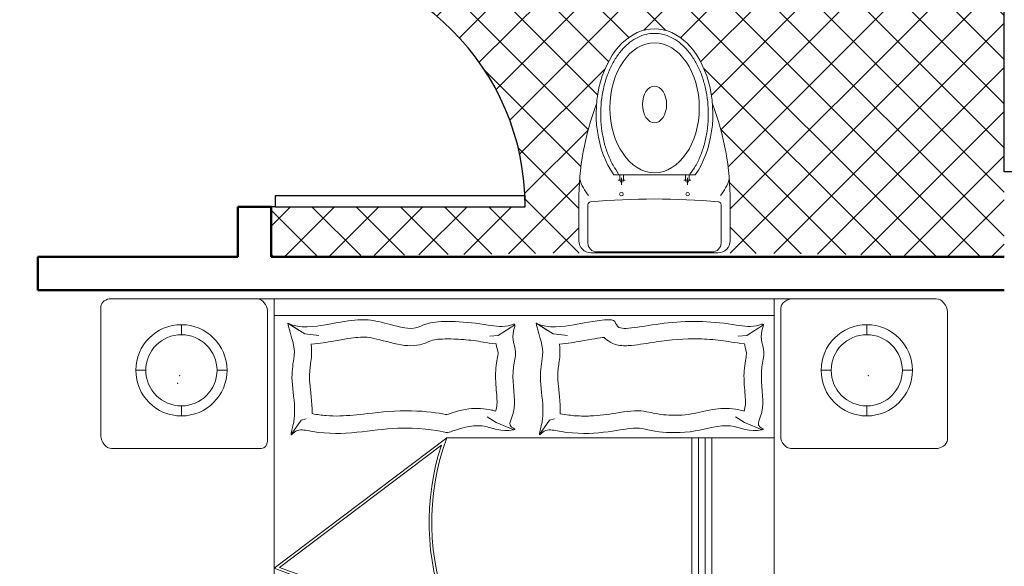
# Model space of a CAD drawing. Units: inches. Extents: x -466983 to 1020, y 324 to 318697.
# Tile 46 of 97: x 491 to 609, y 973 to 1038. Entities that reach past the tile are written whole.
import ezdxf

# ---------------------------------------------------------------- set-up
doc = ezdxf.new("R2010")
doc.units = ezdxf.units.IN
doc.header["$MEASUREMENT"] = 0
for name, color, linetype, lineweight in [('A-DOOR', 3, 'Continuous', 25), ('A-FLOR-FIXT', 9, 'Continuous', 18), ('A-FLOR-PATT', 252, 'Continuous', 13), ('A-FURN', 8, 'Continuous', 18), ('A-GLAZ', 4, 'Continuous', 25), ('A-WALL', 7, 'Continuous', 50)]:
    doc.layers.add(name, color=color, linetype=linetype, lineweight=lineweight)

# ---------------------------------------------------------------- blocks, each defined once
blk = doc.blocks.new('Ventilator')
for p, q in [((1433.5927409432, 801.6799676286266), (1457.592740943201, 801.6799676286266)), ((1433.5927409432, 792.6799676286266), (1433.5927409432, 801.6799676286266)), ((1457.592740943201, 801.6799676286266), (1457.592740943201, 792.6799676286266)), ((1433.5927409432, 797.9799676286265), (1457.592740943201, 797.9799676286265)), ((1457.592740943201, 796.3799676286266), (1433.5927409432, 796.3799676286266)), ((1457.592740943201, 792.6799676286266), (1433.5927409432, 792.6799676286266))]:
    blk.add_line(p, q)
blk = doc.blocks.new('A$C05F852CF')
for p, q in [((0.0305768516066087, 3.078317078245163), (0.4691515062860628, 3.078317078245164)), ((0.4691515062860671, 3.078317078245163), (2.07682031226372, 3.078317078245163)), ((0.5200001058256021, 3.078317078245163), (0.5200001058256021, 1.078317078245163)), ((2.020000105825602, 3.078317078245163), (2.020000105825602, 1.078317078245163)), ((2.076820312263923, 3.078317078245163), (2.506611773352182, 3.078317078245163)), ((1.058288035e-07, 3.054839612522671), (1.058288035e-07, 2.665863151727971)), ((2.040000105829676, 3.050045752684985), (2.040000105829677, 2.664204404880085)), ((0.5000001058288034, 3.042296501208146), (0.5000001058288035, 2.649646432748242)), ((0.5200001058256021, 3.028317078242253), (2.020000105825602, 3.028317078242253)), ((2.540000105829677, 2.654697021141195), (2.540000105829677, 3.039330964775836)), ((0.2417833150248043, 2.970224330108612), (0.2417833150248043, 3.000224330113269)), ((0.5608743282500654, 3.00448058915208), (0.5953432699752739, 2.982949469987943)), ((0.5608743282500654, 3.00448058915208), (0.6121479649955291, 2.972452371068357)), ((1.242739223729586, 2.999473446026968), (1.192734207375906, 2.968208048550877)), ((2.298216896626399, 2.970224330108612), (2.298216896626399, 3.000224330113269)), ((0.6121479649955291, 2.972452371068357), (0.6546239254166722, 2.968208048550877)), ((1.192734207375906, 2.968208048550877), (1.167248631121765, 2.9660858872885)), ((0.1349139653742895, 2.863354980458097), (0.1049139653742895, 2.863354980458097)), ((0.3486526646753191, 2.863354980458097), (0.3786526646753191, 2.863354980458097)), ((2.191347546975884, 2.863354980458097), (2.161347546975885, 2.863354980458097)), ((2.405086246276914, 2.863354980458097), (2.435086246276914, 2.863354980458097)), ((0.2417833150248043, 2.726485630810202), (0.2417833150248043, 2.756485630807583)), ((2.298216896626399, 2.726485630810202), (2.298216896626399, 2.756485630807583)), ((1.186362799460766, 2.707182858976011), (1.158753439034626, 2.724160116791608)), ((0.571055790554965, 2.671151427624863), (0.6015289887363906, 2.713549342755868)), ((0.6015289887363906, 2.713549342755868), (0.6163955887241173, 2.717793665280623)), ((1.239669649243296, 2.685196542661287), (1.186362799460766, 2.707182858976011)), ((1.037932771781925, 2.66077471069002), (0.5200001058256021, 2.269743772885703)), ((2.020000105825602, 2.66077471069002), (1.037932771781925, 2.66077471069002)), ((1.773666079527174, 2.66077471069002), (1.773666079527174, 1.078317078245163)), ((1.793666079523973, 2.66077471069002), (1.793666079523973, 1.078317078245163)), ((1.813666079528047, 2.66077471069002), (1.813666079528047, 1.078317078245163)), ((1.833666079524846, 2.66077471069002), (1.833666079524846, 1.078317078245163)), ((0.0321551649834042, 2.628317078240798), (0.4826422377176051, 2.628317078240797)), ((2.070734587595952, 2.628317078240797), (2.505643211553573, 2.628317078240797)), ((0.5200001058256021, 1.459699989092769), (2.020000105825602, 1.459699989092769)), ((0.5200001058256021, 1.43969998909597), (2.020000105825602, 1.43969998909597)), ((0.5200001058256021, 1.419699989099171), (2.020000105825602, 1.419699989099171)), ((0.5200001058256021, 1.399699989095097), (2.020000105825602, 1.399699989095097)), ((0.5200001058256021, 1.078317078245163), (2.020000105825602, 1.078317078245163)), ((0.7260346108741942, 0.4345828151708702), (0.7377091281887261, 0.4443788983408013))]:
    blk.add_line(p, q)
for points in [[(1.340512920731271, 2.982949469987943), (1.306043979006062, 3.00448058915208), (1.357317615751526, 2.972452371068357), (1.399793576172669, 2.968208048550877)], [(1.987908874485583, 2.999473446026968), (1.937903858124627, 2.968208048550877), (1.912418281870486, 2.9660858872885)], [(1.984839299999293, 2.685196542661287), (1.931532450216764, 2.707182858976011), (1.903923089790623, 2.724160116791608)], [(1.316225441310962, 2.671151427624863), (1.346698639485111, 2.713549342755868), (1.361565239480114, 2.717793665280623)]]:
    blk.add_lwpolyline(points)
for points in [[(1.035294798241981, 2.137877542112184, -0.1730319288328975), (1.021984534024188, 2.638847447216473), (0.5360171556477639, 2.271949793912513, 0.0538879536169309)], [(1.708050559093439, 1.775878924940549, 0.1013919188288575), (1.728157492045764, 1.750061837442286, -0.2237680031452591), (1.734490876633178, 1.736012066440117, -0.2555795276033393), (1.73151803809566, 1.730786319379855, -0.0815627079958122), (1.715055393804573, 1.724012337983466, -0.0718052278729777), (1.696654411599312, 1.722458737045573, 0.0699853124223817), (1.677774125455085, 1.720933512357767, 0.0354599114355874), (1.614797373554905, 1.702055242289732, 0.0294323486882548), (1.54253181370024, 1.669698476292178, 0.001553930981739), (1.507841381839936, 1.651508640737627, -0.0015200052493194), (1.472377942403747, 1.632910412866881, -0.0047351393002262), (1.435637173695639, 1.614224569329063, 0.003820482062427), (1.390058392027433, 1.591148680402633, 0.2960011454759293), (1.369157347081392, 1.554552950265695, -0.6497743315171824), (1.346832187453866, 1.543071524364048, -0.0231899320323143), (1.341607642712404, 1.547689019153187, 0.0288000576854015), (1.337358154039801, 1.551360714168372, 0.0057266563932194), (1.329792250482655, 1.557035683033763, -0.0043580795685463), (1.319830170733231, 1.564465434900571, -0.0275279631909796), (1.300139484251123, 1.581205024032326, -0.0462141900082825), (1.289988230316169, 1.592806604542285, -0.1941210974269485), (1.285597174805949, 1.61052060476509, 0.1337189317945981), (1.282347392942978, 1.636304919732166, 0.0115049885998871), (1.262248195883971, 1.682017285758821, 0.0088817842639035), (1.233822341202832, 1.740117109611183, 0.0124257132779513), (1.193744434042254, 1.813894083333623, -0.033612369588165), (1.180083210426986, 1.841797703870053), (1.155232457866077, 1.902584981879044), (1.136061875891755, 1.949478028393059, 0.224341071481397), (1.120380687047856, 1.963834925633848, -0.722771521635921), (1.120197630008879, 1.973398278848949, -0.1035130421165991), (1.124231807418808, 1.97393370871293, 0.0534647388739861), (1.132045497836501, 1.974187654123627, 0.0301092765073397), (1.156931902511403, 1.97921985894508, -0.0314364784170881), (1.180782283804338, 1.983976772955894, -0.0532399639377359), (1.197102041045038, 1.984427853473678, 0.0551795233422178), (1.212849660231511, 1.984924081265458, 0.0562710065808877), (1.240173079634912, 1.992022438719103, 0.0108003168714398), (1.37589919497303, 2.047527127645597, 0.0045599262081994), (1.467518199665537, 2.08832242005046, 0.0112502044116702), (1.504115679717903, 2.10602511197999, 0.0693939606021616), (1.523450236066789, 2.119584464602007, -0.0797562576808959), (1.540538561194231, 2.131050544499311, -0.1063994920026711), (1.556160884733792, 2.134540918040703, -0.3286420828127689), (1.560758069905846, 2.131208477514896, -0.2995467620412478), (1.558739430321109, 2.124014460027718, 0.1899166395855367), (1.553562506110245, 2.114077400326368, 0.0335175219245665), (1.553139912342055, 2.102935661711667, 0.0756271023396346), (1.554028972653962, 2.098051728963763, 0.0534886288518014), (1.55787110568871, 2.089846036281636, 0.0178378665464654), (1.572733087595266, 2.067184354551788, 0.0383935758418631), (1.593239248720917, 2.042483627130348, -0.0595290829391222), (1.605807381512724, 2.025975353424011, -0.0359425919331862), (1.619326798747338, 1.998683789839922, -0.0112450065700176), (1.654088856282072, 1.907874325597662, -0.006202709412992), (1.668419968066657, 1.866129904310976, 0.0107832106742137), (1.67688376537216, 1.842192375839789, 0.0194848354522239), (1.682775803493053, 1.828271519536226, 0.005061623460185)], [(1.695259182866416, 1.769547813629049, 0.0985872314327748), (1.718081561207793, 1.739905989662399, -0.0403778893328424), (1.71183503166025, 1.737916709378077, -0.0718052278729781), (1.697497903411904, 1.736706220956143, 0.0699853124223817), (1.674654559801433, 1.734860844706513, 0.0354599114355874), (1.609741097926352, 1.715402015419892, 0.0294323486882547), (1.535943288060523, 1.682359187414175, 0.001553930981739), (1.50117428856039, 1.664128155126926, -0.0015200052493194), (1.465787698753773, 1.645570229802914, -0.0047351393002262), (1.429287879954427, 1.627006930034647, 0.003820482062427), (1.383514509072797, 1.603832523357192, 0.2898135525162437), (1.354853178569346, 1.554951448117944, -0.0182793572286215), (1.35154491067881, 1.557933675398455, 0.0288000576854021), (1.346052337980832, 1.562679435024519, 0.0057266563932193), (1.338224905351514, 1.568550569402397, -0.0043580795685465), (1.328462264060592, 1.575831579409929, -0.0275279631909798), (1.309968032010976, 1.591554030030593, -0.0462141900082822), (1.301550432054356, 1.60117426653267, -0.1941210974269471), (1.299728996962296, 1.608522135660689, 0.1337189317945981), (1.295541371992653, 1.641747455267798, 0.0115049885998871), (1.275177841475791, 1.688061004902677, 0.0088817842639034), (1.246529163101812, 1.746616259820824, 0.0124257132779513), (1.206112688769413, 1.821016481189961, -0.0336123695881646), (1.193294292057559, 1.847198592534913), (1.168443539497244, 1.907985870542451), (1.149272957522402, 1.954878917057737, 0.0514173808819106), (1.145486925332716, 1.961962889445687, 0.0172081957648061), (1.160597165040831, 1.965426087640239, -0.031436478417088), (1.182689249433297, 1.969832312615894, -0.0532399639377359), (1.195979299991558, 1.970199651593374, 0.0551795233422181), (1.214865982280068, 1.970794795309813, 0.0562710065808877), (1.245288872283408, 1.978698364950264, 0.0108003168714398), (1.381585630304949, 2.034436416074573, 0.0045599262081997), (1.473442444961096, 2.075337598376756, 0.0112502044116702), (1.510618033905799, 2.093319929327427, 0.0693939606021616), (1.533180597587688, 2.109143088213213, -0.0381608677403329), (1.539212311339161, 2.113959948097047, 0.0293614558111777), (1.538873523984414, 2.102520403419968, 0.0756271023396326), (1.540531433152462, 2.093412903290674, 0.0534886288518001), (1.545664760729809, 2.082449589907588, 0.0178378665464654), (1.561085038110327, 2.058936614290585, 0.0383935758418633), (1.582989208528954, 2.032551912661889, -0.0595290829391216), (1.593505968643746, 2.018738122071704, -0.0359425919331862), (1.606115717130862, 1.99328290114058, -0.0112450065700176), (1.640648295649741, 1.903072908503876, -0.0062027094129919), (1.654864430545357, 1.861663397988524, 0.0107832106742138), (1.663533420481039, 1.837145538462979, 0.0194848354522239), (1.669858875879018, 1.822200666446777, 0.005061623460185)]]:
    blk.add_lwpolyline(points, format="xyb", close=True)
for points in [[(1.270020360572594, 1.665009431050252, 0.0256263766809095), (1.257496937469981, 1.661962907224936, 0.0108003168915285), (1.117915806080817, 1.617024549173869, 0.0045599250600183), (1.023439488402936, 1.583371629054553, 0.0112502042554101), (0.9855927851847837, 1.568526107768631, 0.0693939618380823), (0.9652758158050374, 1.556488585590853, -0.0797562567609452), (0.9473589151510481, 1.546366011015306, -0.1063994945831262), (0.9315150200727321, 1.5440833152102, -0.3286420812263602), (0.9271867815419792, 1.54775831472709, -0.2995467631228521), (0.9297508853421131, 1.554776445874623, 0.1899166395519681), (0.9356742299125951, 1.564287475604295, 0.0335175234261574), (0.9369495655297574, 1.575364047566859, 0.075627101586891), (0.9364374612317099, 1.580301757141754, 0.0534886298074961), (0.9332355752115681, 1.588777800893726, 0.0178378665269371), (0.9201542714773111, 1.612511950054128, 0.0383935757768284), (0.9016016807480021, 1.63871175657932, -0.0595290839550855), (0.8903358353981968, 1.656134782393036, -0.0359425913009802), (0.8789480177289066, 1.684382282033313, -0.0112450075583744), (0.8512485241325798, 1.777589041382892, -0.0062027096904869), (0.8401591725715132, 1.820309097441429, 0.0107832125180045), (0.8335550214589964, 1.844824938410538, 0.0194848341872523), (0.8287473142423458, 1.859156449308979, 0.0050616244400538), (0.8075626644720159, 1.913332163710765, 0.1013919188235688), (0.7894936926428668, 1.940614447702458, -0.22376800337822), (0.7842558173954927, 1.955108325059244, -0.2555795277823594), (0.7876204503391627, 1.960090839085296, -0.0815627097533239), (0.8045538741787872, 1.965583074885499, -0.0718052258191368), (0.8230198047757069, 1.965721718523918, 0.0699853122038087), (0.8419614541001006, 1.96579533206703, 0.0354599118842221), (0.9061999169328895, 1.979791065284685, 0.0294323472364991), (0.980732947874111, 2.006513679583421, 0.0015539321746028), (1.016715544742657, 2.021991080197058, -0.0015200050660023), (1.05350014010862, 2.037816406693342, -0.0047351399682821), (1.091565063355451, 2.053631204585071, 0.0038204811652429), (1.138778458583519, 2.07314571145658, 0.2960011456451315), (1.162422996298041, 2.10803178119455, -0.6497743308183526), (1.18556250232168, 2.117768267051117, -0.023189931893098), (1.190417758999585, 2.112763908071101, 0.0288000584975066), (1.194373321091643, 2.108777302019709, 0.0057266569232023), (1.201481997667391, 2.102539119626516, -0.0043580803905699), (1.210845298395146, 2.094367658855894, -0.0275279623196554), (1.229195014547529, 2.07616807397338, -0.046214191426687), (1.238427176317387, 2.063822554404071, -0.1941210967300704), (1.24144758291114, 2.045824101341992, 0.1337189329089291), (1.242711504870895, 2.019866549455296, 0.005779060601493), (1.250747094455965, 1.996102607779307)], [(1.267433777013181, 1.678650745174671, 0.0256263766809096), (1.25352836721457, 1.6752680308876, 0.0108003168915285), (1.113376341331941, 1.630145872481547, 0.0045599250600184), (1.018661464651108, 1.596407976494609, 0.0112502042554101), (0.9802331745365827, 1.581334325413979, 0.0693939618380822), (0.9566164053315807, 1.567341717664273, -0.0421754501329271), (0.9494714401999663, 1.562566648678462, 0.0314567403863147), (0.950818198592405, 1.574703076671485, 0.0756271015868911), (0.9498752735948789, 1.583794759352339, 0.0534886298074966), (0.9456266121275149, 1.595041830722721, 0.0178378665269371), (0.9320672656192937, 1.619643319917204, 0.0383935757768284), (0.9122842399252132, 1.647580735944291, -0.0595290839550849), (0.9028072117943391, 1.662237293051497, -0.0359425913009799), (0.8921648024522767, 1.688635806116587, -0.0112450075583744), (0.8646431932534301, 1.781243997565097, -0.006202709690487), (0.8536403913351593, 1.823630634163732, 0.0107832125180045), (0.8468804852507327, 1.848724666642867, 0.0194848341872522), (0.8417287394599854, 1.864081737612187, 0.0050616244400538), (0.8204417169625553, 1.918519250802461, 0.1002374450930622), (0.7996032399862063, 1.950139962323341, -0.0442087188515421), (0.806640704233721, 1.951856421765647, -0.0718052258191371), (0.8211393199436285, 1.951965278492165, 0.0699853122038086), (0.8439488047114903, 1.952053923729516, 0.0354599118842221), (0.910109066083358, 1.966468362162935, 0.0294323472364991), (0.9861794565215773, 1.993742171876655, 0.0015539321746028), (1.022241331845213, 2.00925367298648, -0.0015200050660023), (1.05894838186196, 2.025045638222023, -0.0047351399682822), (1.096770458708799, 2.040759540948764, 0.0038204811652431), (1.144179941304543, 2.06035509575735, 0.2942870031128779), (1.176296866445577, 2.107421377421802, -0.0218403622568167), (1.180015238936497, 2.103568069779355, 0.0288000584975063), (1.185096443349676, 2.098446987169159, 0.0057266569232022), (1.192444163039438, 2.091999033726075, -0.0043580803905699), (1.201625109260011, 2.083986715841735, -0.0275279623196552), (1.218890166936317, 2.066862915121399, -0.0462141914266873), (1.226588508356947, 2.05656846545553, -0.1941210967300651), (1.227889447910251, 2.048816231160124, 0.1337189329089299), (1.22950820338519, 2.015571354997711, 0.005779060601493), (1.237646599208447, 1.991503380689822, 0.005779060601493)]]:
    blk.add_lwpolyline(points, format="xyb")
for centre, radius in [((0.2417833150248043, 2.863354980458097), 0.1368693496505148), ((2.298216896626399, 2.863354980458097), 0.1368693496505148), ((0.2417833150248043, 2.863354980458097), 0.1068693496505148), ((2.298216896626399, 2.863354980458097), 0.1068693496505148)]:
    blk.add_circle(centre, radius)
for centre, radius, start, end in [((1.730780082035789, 2.407017656099047), 0.7378550251104214, 159.8846174586709, 202.2193637034114), ((1.40584522550477, 4.514464091946545), 2.413191017483698, 248.464074582217, 261.4655058976137)]:
    blk.add_arc(centre, radius, start, end)
for points in [[(1.058288035e-07, 3.054839612522671), (1.058288035e-07, 3.067689726137004), (0.0177267379922761, 3.078317078245163), (0.0305768516066087, 3.078317078245163)], [(0.5000001058288034, 3.042296501208146), (0.5000001058288034, 3.058104790397429), (0.4849597954753462, 3.078317078245164), (0.4691515062860628, 3.078317078245164)], [(2.040000105829676, 3.050045752684985), (2.040000105829676, 3.065519728870074), (2.061346336078835, 3.078317078245163), (2.076820312263923, 3.078317078245163)], [(2.506611773352182, 3.078317078245163), (2.523721542455991, 3.078317078245163), (2.540000105829677, 3.056440733879645), (2.540000105829677, 3.039330964775836)], [(0.0321551649834042, 2.628317078240798), (0.0156773837697008, 2.628317078240798), (1.058288035e-07, 2.649385370514268), (1.058288035e-07, 2.665863151727971)], [(2.040000105829677, 2.664204404880085), (2.040000105829677, 2.648454595065514), (2.05498477778138, 2.628317078240797), (2.070734587595952, 2.628317078240797)], [(0.5000001058288035, 2.649646432748242), (0.5000001058288035, 2.640479845178462), (0.4918088252873853, 2.628317078240797), (0.4826422377176051, 2.628317078240797)], [(2.505643211553573, 2.628317078240797), (2.52008196177545, 2.628317078240797), (2.540000105829677, 2.640258270919319), (2.540000105829677, 2.654697021141195)]]:
    blk.add_open_spline(points, degree=3)
for points, knots in [([(0.5608743282500654, 3.00448058915208), (0.5649926015757956, 2.981846978706016), (0.583561233303044, 2.936624526169907), (0.577615531939955, 2.888972981483675), (0.568850038027449, 2.835056739670108), (0.5831844526110217, 2.770926244731526), (0.5807655002863612, 2.708841986364859), (0.5743850803628447, 2.69267683673388), (0.5692655243474292, 2.665138401345757), (0.5802504519451759, 2.679294818459311), (0.5989340893502231, 2.687563487939769), (0.7172179605840939, 2.659836610568163), (0.8680758339905879, 2.702933271801157), (1.048422440333524, 2.678138835668505), (1.032371212037105, 2.673100819083629), (1.143052510538836, 2.711612612161843), (1.202032879395119, 2.675720859246212), (1.245920398971065, 2.686747608633595), (1.222151592133741, 2.694979075698938), (1.235874692996731, 2.725131493731169), (1.24678286496055, 2.780968112114351), (1.22880829625501, 2.849214346417284), (1.25148706651089, 2.925020729671814), (1.227919394332275, 2.960895142656227), (1.247080047731287, 3.005764387140516), (1.209778335498413, 2.990212765405885), (1.117656181813799, 3.009504931840638), (0.9559744755824794, 3.015881985804298), (0.9531522539109573, 2.975810997435473), (0.7998968530228013, 3.020986756855563), (0.7569283034463297, 3.015103121600986), (0.5985546251031338, 2.986850236149621), (0.5610488986203565, 3.004875976599578)], [16.81603238654801, 16.81603238654801, 16.81603238654801, 16.81603238654801, 79.03884518756725, 88.51389547092393, 147.5652660998466, 227.1968623982579, 259.6854484034709, 283.9553011869364, 296.5113041396114, 302.4325582064448, 320.2309418964503, 354.3225591584033, 575.2795485590284, 734.7235597353396, 845.7404214628034, 943.0331034920418, 1029.53396696452, 1032.845074190681, 1043.313583943025, 1065.311533561496, 1104.921834519419, 1208.530020162994, 1248.510714137047, 1303.102727458275, 1321.013260208933, 1329.647833410585, 1389.371623582993, 1571.817643787636, 1750.274160612537, 1823.189072856133, 1967.937032714809, 2020.91232922514, 2020.91232922514, 2020.91232922514, 2020.91232922514]), ([(1.306043979006062, 3.00448058915208), (1.310162252324516, 2.981846978706016), (1.328730884059041, 2.936624526169907), (1.322785182695952, 2.888972981483675), (1.31401968877617, 2.835056739670108), (1.328354103367018, 2.770926244731526), (1.325935151042358, 2.708841986364859), (1.319554731111566, 2.69267683673388), (1.31443517509615, 2.665138401345757), (1.325420102701173, 2.679294818459311), (1.344103740098944, 2.687563487939769), (1.462387611340091, 2.659836610568163), (1.613245484739309, 2.702933271801157), (1.643592091088066, 2.678138835668505), (1.777540862793102, 2.673100819083629), (1.888222161287558, 2.711612612161843), (1.947202530151116, 2.675720859246212), (1.991090049727063, 2.686747608633595), (1.967321242889738, 2.694979075698938), (1.981044343745452, 2.725131493731169), (1.991952515709272, 2.780968112114351), (1.973977947003731, 2.849214346417284), (1.996656717266887, 2.925020729671814), (1.973089045080996, 2.960895142656227), (1.992249698480009, 3.005764387140516), (1.95494798625441, 2.990212765405885), (1.862825832569797, 3.009504931840638), (1.7011441263312, 3.015881985804298), (1.548321904665499, 2.975810997435473), (1.545066503778798, 3.020986756855563), (1.502097954202326, 3.015103121600986), (1.343724275859131, 2.986850236149621), (1.306218549376353, 3.004875976599578)], [16.81603238654801, 16.81603238654801, 16.81603238654801, 16.81603238654801, 79.03884518756725, 88.51389547092393, 147.5652660998466, 227.1968623982579, 259.6854484034709, 283.9553011869364, 296.5113041396114, 302.4325582064448, 320.2309418964503, 354.3225591584033, 575.2795485590284, 734.7235597353396, 845.7404214628034, 943.0331034920418, 1029.53396696452, 1032.845074190681, 1043.313583943025, 1065.311533561496, 1104.921834519419, 1208.530020162994, 1248.510714137047, 1303.102727458275, 1321.013260208933, 1329.647833410585, 1389.371623582993, 1571.817643787636, 1750.274160612537, 1823.189072856133, 1967.937032714809, 2020.91232922514, 2020.91232922514, 2020.91232922514, 2020.91232922514]), ([(1.186008792049375, 2.94299214351074), (1.155725921251891, 2.945585073046202), (1.138656601401412, 2.950208126398367), (1.097630905252152, 2.95509280500171), (1.077589870855775, 2.956659449204214), (1.034238225660662, 2.958226127717206), (1.012323327727554, 2.957004601752403), (0.991001711516253, 2.953273250088436), (0.9901760228479028, 2.951676768007356), (0.9620368334136054, 2.940252037519872), (0.9370877461655887, 2.935037325494899), (0.8850511336414232, 2.94132938915891), (0.8522462034232987, 2.951314821397172), (0.803295939310399, 2.96285187557315), (0.7937503361772829, 2.963996187832593), (0.7550144806336718, 2.960828646016758), (0.7318586182640057, 2.957210255508529), (0.679441891670091, 2.948089555791339), (0.6579881949560275, 2.943409279898279), (0.630985700249326, 2.941762475625111)], [1364.380335490081, 1364.380335490081, 1364.380335490081, 1364.380335490081, 1423.602309547691, 1423.602309547691, 1482.824283605301, 1482.824283605301, 1566.205036495643, 1566.205036495643, 1649.585789385986, 1649.585789385986, 1732.966542276328, 1732.966542276328, 1816.347295166671, 1816.347295166671, 1899.728048057014, 1899.728048057014, 1960.499853060085, 1960.499853060085, 1990.525565429441, 1990.525565429441, 1990.525565429441, 1990.525565429441]), ([(1.510355574678164, 2.962131737273937), (1.496402554093968, 2.960566078706099), (1.473180590099924, 2.956790270249104), (1.422578285991909, 2.947958552952412), (1.401696155951149, 2.943524922981268), (1.375888251815216, 2.941975038078444)], [1904.396500054124, 1904.396500054124, 1904.396500054124, 1904.396500054124, 1961.927875749907, 1961.927875749907, 1990.619444948187, 1990.619444948187, 1990.619444948187, 1990.619444948187]), ([(1.931373767935067, 2.94320464204133), (1.899671311434888, 2.945891083962288), (1.88221689097919, 2.950718490397115), (1.838682954929346, 2.955652880867252), (1.816795986262647, 2.957169928676467), (1.751472258998956, 2.958725448706285), (1.708807917427409, 2.955142722863579), (1.640333479281332, 2.944746536498916), (1.615392287461663, 2.940198542969911), (1.579493331147493, 2.936988078909458), (1.567546271042127, 2.936091768500583), (1.539405034045934, 2.941198470052663), (1.5201082499519, 2.950733332609488), (1.510355574678187, 2.962131737273942)], [1364.265661087181, 1364.265661087181, 1364.265661087181, 1364.265661087181, 1426.240794565023, 1426.240794565023, 1488.215928042865, 1488.215928042865, 1612.166194998548, 1612.166194998548, 1689.928639661805, 1689.928639661805, 1733.064361503359, 1733.064361503359, 1768.978829433574, 1768.978829433574, 1768.978829433574, 1768.978829433574]), ([(0.6309857002492723, 2.941762475624982), (0.6331564334752285, 2.928751157475458), (0.6329999809455203, 2.910376883670986), (0.6307844219696133, 2.892950992011628), (0.6298480683836976, 2.88648431095065), (0.6280366860877277, 2.872562196049626), (0.6272625999342161, 2.865990559597485), (0.6256841353987236, 2.847428671628844), (0.6257494163208535, 2.83751285108547), (0.6289829528156191, 2.801318580102345), (0.6345320734627763, 2.769590933476876), (0.6337228367630585, 2.733309880517507)], [67.28536243525942, 67.28536243525942, 67.28536243525942, 67.28536243525942, 87.39955824583018, 87.39955824583018, 107.5137540564009, 107.5137540564009, 127.6279498669717, 127.6279498669717, 167.8563414881131, 167.8563414881131, 238.1272680512623, 238.1272680512623, 238.1272680512623, 238.1272680512623]), ([(1.184532074545908, 2.741151129000606), (1.18898166794339, 2.755206550563011), (1.189354860725254, 2.765005834716451), (1.187413425890239, 2.799822569981758), (1.184324887423806, 2.821896583953417), (1.184425468230181, 2.866418567383826), (1.188231061791394, 2.890075729955087), (1.192008110665926, 2.910542534993727), (1.192192726159281, 2.914423416697752), (1.192086062290282, 2.915789359669391), (1.190808194988107, 2.921220065210955), (1.187543579250811, 2.935072419567428), (1.18672591971923, 2.938807649824122), (1.186008792049374, 2.94299214351074)], [1072.516900511537, 1072.516900511537, 1072.516900511537, 1072.516900511537, 1129.100963921242, 1129.100963921242, 1185.685027330947, 1185.685027330947, 1226.035089289856, 1226.035089289856, 1249.281274409203, 1249.281274409203, 1272.52745952855, 1272.52745952855, 1279.68927491123, 1279.68927491123, 1279.68927491123, 1279.68927491123]), ([(1.375888251815172, 2.941975038078342), (1.378074137039331, 2.928979344370601), (1.377968860976706, 2.910637565443015), (1.375735790312178, 2.893015133736763), (1.37480390116772, 2.88660606446792), (1.37298778010343, 2.872656318465669), (1.37221091417058, 2.866070180858095), (1.370625496709551, 2.847462614183982), (1.370689547662139, 2.837514257962978), (1.37393087155791, 2.801238188465308), (1.379492518843283, 2.769438786188064), (1.378659813172273, 2.733119478683537)], [67.15622801377181, 67.15622801377181, 67.15622801377181, 67.15622801377181, 87.29721209066957, 87.29721209066957, 107.4381961675674, 107.4381961675674, 127.5791802444651, 127.5791802444651, 167.8611483982607, 167.8611483982607, 238.2535697831694, 238.2535697831694, 238.2535697831694, 238.2535697831694]), ([(1.929853198197663, 2.740873894614667), (1.934365908758641, 2.755026217031627), (1.934751701761907, 2.764815030887031), (1.932835938875, 2.79960316592369), (1.929746498563042, 2.821657635936312), (1.929805814653183, 2.866185379441856), (1.933600746470114, 2.88991221701699), (1.937403886615359, 2.910503728082434), (1.937594356706148, 2.914393286831795), (1.937478304969509, 2.915863471904236), (1.936169207211093, 2.921368445863724), (1.93289467066463, 2.935308900229952), (1.932083262228118, 2.939035512649967), (1.931373767950089, 2.943204642135211)], [1072.238498285051, 1072.238498285051, 1072.238498285051, 1072.238498285051, 1128.864868567103, 1128.864868567103, 1185.491238849155, 1185.491238849155, 1225.989552664987, 1225.989552664987, 1249.32640120519, 1249.32640120519, 1272.663249745394, 1272.663249745394, 1279.788507909373, 1279.788507909373, 1279.788507909373, 1279.788507909373]), ([(1.03809723815708, 2.73039727020292), (1.049717200660217, 2.734487788763535), (1.074192496521652, 2.74352113186204), (1.125142067689975, 2.75041210718968), (1.152757231246774, 2.748989383813843), (1.176896856726861, 2.743194484257486), (1.18086569021346, 2.742138176736147), (1.184532074545908, 2.741151129000606)], [843.6450298341101, 843.6450298341101, 843.6450298341101, 843.6450298341101, 911.2757195712669, 911.2757195712669, 959.0880622759533, 959.0880622759533, 969.4799795511734, 969.4799795511734, 969.4799795511734, 969.4799795511734]), ([(1.37865981314566, 2.733119478685147), (1.398350924522489, 2.729609953669208), (1.410621471748096, 2.727818570031879), (1.440144629954641, 2.725836663619492), (1.45453272438222, 2.72579428596297), (1.496194066974801, 2.72756283296527), (1.521854810648972, 2.731279274356243), (1.576694937727594, 2.739864181267917), (1.6067435507169, 2.743633804836029), (1.652654114968593, 2.737068097937112), (1.661975420857501, 2.732604969096766), (1.708415029150631, 2.728170445544914), (1.736441496722281, 2.727579800786222), (1.784873006914288, 2.733957286540809), (1.807601793062205, 2.740559362958333), (1.856301372606796, 2.748907303561592), (1.881197134759921, 2.750793202553537), (1.914047432134626, 2.745130255701714), (1.922553922867449, 2.74284011529716), (1.929853198197665, 2.74087389461467)], [345.2679180365509, 345.2679180365509, 345.2679180365509, 345.2679180365509, 387.1674142554489, 387.1674142554489, 429.0669104743468, 429.0669104743468, 512.8659029121428, 512.8659029121428, 629.3175453119198, 629.3175453119198, 745.7691877116971, 745.7691877116971, 834.6228130435273, 834.6228130435273, 901.4144086089123, 901.4144086089123, 948.9218778206058, 948.9218778206058, 969.6795111477606, 969.6795111477606, 969.6795111477606, 969.6795111477606]), ([(0.6337228367630439, 2.733309880517508), (0.6515219447508598, 2.730130838331354), (0.6627469292146047, 2.728404560298634), (0.6898215070493534, 2.726294045804654), (0.7032356687061024, 2.726036490933712), (0.7435886058342663, 2.726989827329198), (0.7706550133649461, 2.729971405875143), (0.8408783579177043, 2.738316880491805), (0.888120323933067, 2.743221924747295), (0.9755155714750383, 2.740575358042937), (1.012451770127618, 2.735676002774785), (1.035649434709067, 2.730930674356534), (1.036885983111078, 2.730667355489783), (1.038097238090126, 2.730397270179416)], [345.40469962997, 345.40469962997, 345.40469962997, 345.40469962997, 383.3860561782741, 383.3860561782741, 421.3674127265782, 421.3674127265782, 497.3301258231863, 497.3301258231863, 611.5614694743621, 611.5614694743621, 725.792813125538, 725.792813125538, 732.4347682895597, 732.4347682895597, 732.4347682895597, 732.4347682895597])]:
    blk.add_open_spline(points, degree=3, knots=knots)
for p in [(0.2366049805932562, 2.847463833648362), (2.303395231057947, 2.847463833648362), (0.2308577250878443, 2.824418416894332), (2.020000105825602, 1.078317078245163), (2.020000105825602, 1.078317078245163)]:
    blk.add_point(p)
blk = doc.blocks.new('A$C005B7AE8')
for p, q in [((0.4599999173160541, 0.7399999669141835), (0.0399999173159813, 0.7399999669141835)), ((0.439999917316527, 0.7369231961274636), (0.0599999173164179, 0.7369231961274636)), ((-8.26839823e-08, 0.6999999669133103), (-8.26839823e-08, 0.5690287834004267)), ((0.0299999173166725, 0.7069231961286278), (0.029999917315763, 0.5811477270617617)), ((0.4699999173162724, 0.7069231961286278), (0.4699999173162724, 0.5811477270617617)), ((0.4999999173160177, 0.6999999669133103), (0.4999999173160177, 0.5690287833785987)), ((0.1298495880610062, 0.5003783992360696), (0.1533971911394474, 0.5003783992360696)), ((0.135565754210802, 0.4819999669125537), (0.135565754210802, 0.5011511907214299)), ((0.1415172819179133, 0.4916755243175431), (0.1415172819179133, 0.5154492432702682)), ((0.1478168830781215, 0.5011511907214299), (0.1478168830781215, 0.4819999669125537)), ((0.3701502465710291, 0.5003783992360696), (0.3466026434934974, 0.5003783992360696)), ((0.3521829515548234, 0.5011511907214299), (0.3521829515548234, 0.4819999669125537)), ((0.3584825527150315, 0.4916755243175431), (0.3584825527150315, 0.5154492432702682)), ((0.3644340804221429, 0.4819999669125537), (0.3644340804221429, 0.5011511907214299)), ((0.3846918195813487, 0.4819999669125537), (0.1153080150515962, 0.4819999669125537))]:
    blk.add_line(p, q)
for centre in [(0.1407590817070741, 0.546016981927096), (0.3592407529249613, 0.546016981927096)]:
    blk.add_circle(centre, 0.0058207128015492)
for centre, radius, start, end in [((0.0399999173159813, 0.6999999669133103), 0.04, 90, 180), ((0.0599999173164179, 0.7069231961286278), 0.03, 90, 180), ((0.439999917316527, 0.7069231961286278), 0.03, 0, 90), ((0.4599999173160541, 0.6999999669133103), 0.04, 0, 90), ((0.9162347733818023, 0.5697843573143473), 0.9162351676084766, 179.9527510438183, 200.6123382500767), ((0.0399999173159813, 0.5811477270617617), 0.01, 180, 265.0114580301616), ((0.2499999173160177, 2.986999966909934), 2.424999999999394, 265.0114580301616, 274.9885419698384), ((-0.4162349387497671, 0.5697843573143473), 0.9162351676084766, 339.3876617499233, 0.0472489561816761), ((0.4599999173160541, 0.5811477270617617), 0.01, 274.9885419698384, 0), ((0.1538218116911594, 0.4497837234594045), 0.1578971577643038, 140.181504794802, 162.8477667450203), ((0.346178022940876, 0.4497837234594045), 0.1578971577643038, 17.15223325497964, 39.81849520519793), ((0.141691318644007, 0.5005983719747747), 0.0061504591858251, 5.156848388262675, 174.8431516117373), ((0.3583085159880284, 0.5005983719747747), 0.0061504591858251, 5.156848388262675, 174.8431516117373)]:
    blk.add_arc(centre, radius, start, end)
blk.add_ellipse((0.2499999173160177, 0.2809999669116223), major_axis=(4.3e-15, -0.2809999999999999), ratio=0.6859192225533541, start_param=3.915332106759934, end_param=8.65103850759918)
for centre, major_axis, ratio in [((0.2497273054386824, 0.2607283879333408), (4.6e-15, -0.2143896387416461), 0.687861093389952), ((0.2499999173160177, 0.2495750337038771), (4e-16, -0.0607231097518234), 0.6571642650459009)]:
    blk.add_ellipse(centre, major_axis=major_axis, ratio=ratio)
blk.add_open_spline([(0.1330304284401791, 0.4805691871661111), (0.123297561966865, 0.467275065217109), (0.1192040598116364, 0.4608387557527749), (0.1089923119561718, 0.4430896997000673), (0.103240873932009, 0.4312752909245319), (0.0930943572666365, 0.4063656141879619), (0.0886993987696769, 0.3932708291395102), (0.0814055876480779, 0.3661625228414778), (0.0785067868491751, 0.352149423713854), (0.0742960000825406, 0.3235936370911077), (0.0729840366493591, 0.3090513401839416), (0.0719875980385041, 0.2798412472329801), (0.0723031276866095, 0.2651738304266473), (0.0745519352649353, 0.2361210512899561), (0.076485202062031, 0.2217360707581975), (0.0819094268572371, 0.1936478195857489), (0.0854003532995194, 0.1799449487807578), (0.0938301373234936, 0.1536010168056237), (0.0987689237617815, 0.1409603975334903), (0.1099364044266622, 0.1170889910499682), (0.116164929732804, 0.1058587174047716), (0.1297089136187424, 0.0851097239210503), (0.1370239707930523, 0.0755915829504375), (0.152501027386279, 0.0585057705757208), (0.1606621934961367, 0.0509385682526045), (0.1775722209031301, 0.0379140469667618), (0.1863198251348876, 0.0324565718765371), (0.2041561746218576, 0.023724375780148), (0.2132440667546689, 0.0204483489505947), (0.2315630702087219, 0.0160859502211679), (0.2407950771003016, 0.01499791808601), (0.259256859623747, 0.0150020215223776), (0.2684887415816775, 0.0160941591893789), (0.2868071874390807, 0.0204647859718534), (0.2958946431490403, 0.0237449365959037), (0.3137296967424845, 0.0324853214769974), (0.3224764393571604, 0.0379468595056096), (0.3393842548493922, 0.0509792925877264), (0.3475440710253679, 0.058550341942464), (0.3630179485271583, 0.0756434699942474), (0.3703311774997928, 0.0851650790282293), (0.3838710834670564, 0.1059204943594523), (0.3900973596782933, 0.1171537218178855), (0.4012600005589775, 0.1410304195233039), (0.4061961965880983, 0.1536733763350639), (0.4146205471060967, 0.1800212940433994), (0.4181086305634381, 0.1937258131365524), (0.423527009337704, 0.2218166234742966), (0.425457273147913, 0.2362025149268447), (0.4277000090169168, 0.2652563529190957), (0.4280124699726003, 0.2799239176820265), (0.427009923148944, 0.3091335394783528), (0.4256949202253964, 0.3236752172670094), (0.4214781782784485, 0.3522290158871328), (0.4185764618305257, 0.3662407460942632), (0.4112770365782126, 0.3933456040758756), (0.406879379678685, 0.4064383096483653), (0.3967277738520352, 0.4313431800474064), (0.3909739452683425, 0.4431548618158559), (0.380770586511062, 0.4608783582370961), (0.376689084062491, 0.467293849651469), (0.3673029200963356, 0.4823032274071011)], degree=3, knots=[3.915332106759953, 3.915332106759953, 3.915332106759953, 3.915332106759953, 4.014440589322762, 4.014440589322762, 4.176504673233075, 4.176504673233075, 4.338568757143389, 4.338568757143389, 4.500632841053702, 4.500632841053702, 4.662696924964015, 4.662696924964015, 4.824761008874329, 4.824761008874329, 4.986825092784642, 4.986825092784642, 5.148889176694956, 5.148889176694956, 5.310953260605269, 5.310953260605269, 5.473017344515582, 5.473017344515582, 5.635081428425896, 5.635081428425896, 5.797145512336209, 5.797145512336209, 5.959209596246522, 5.959209596246522, 6.121273680156836, 6.121273680156836, 6.283337764067149, 6.283337764067149, 6.445401847977462, 6.445401847977462, 6.607465931887776, 6.607465931887776, 6.769530015798089, 6.769530015798089, 6.931594099708402, 6.931594099708402, 7.093658183618716, 7.093658183618716, 7.255722267529029, 7.255722267529029, 7.417786351439342, 7.417786351439342, 7.579850435349656, 7.579850435349656, 7.741914519259969, 7.741914519259969, 7.903978603170283, 7.903978603170283, 8.066042687080596, 8.066042687080596, 8.22810677099091, 8.22810677099091, 8.390170854901225, 8.390170854901225, 8.552234938811539, 8.552234938811539, 8.651038507599205, 8.651038507599205, 8.651038507599205, 8.651038507599205])
blk = doc.blocks.new('*U38')
for p, q in [((0, 0), (-1.1e-15, 5.999999999999999)), ((40, 8e-15), (40, 6.000000000000007))]:
    blk.add_line(p, q)
blk.add_lwpolyline([(0, 0), (1.42e-14, -40), (1.750000000000014, -40), (1.75, 9e-16)], close=True)
blk.add_arc((0, 0), 40, 270, 0)

msp = doc.modelspace()

# ---------------------------------------------------------------- hatches: boundary and pattern name
at = {"layer": 'A-FLOR-PATT', "transparency": 33554572}
h = msp.add_hatch(dxfattribs=at)
h.set_pattern_fill('ANSI37', color=256, scale=30)
h.set_pattern_definition([(45, (-1212.413693079869, -290.0350025265127), (-2.651650429449553, 2.651650429449553), []), (135, (-1212.413693079869, -290.0350025265127), (-2.651650429449553, -2.651650429449552), [])])
h.paths.add_polyline_path([(901.805677520904, 1075.937732818422), (900.6144036774049, 1075.937732818422), (900.6144036774049, 1065.385628316983), (899.390971271441, 1065.385628316983), (898.0910743401043, 1065.385628316983), (892.8355944880973, 1058.709752245277, -0.2583770168556315), (892.18750428989, 1058.350891982691), (879.9847834232776, 1058.350891982691, -0.2017697719240963), (879.438188978411, 1058.580825279484), (874.0812133730635, 1065.385628316983), (872.7813164417267, 1065.385628316983), (871.5578840357629, 1065.385628316983), (871.5578840357629, 1075.937732818422), (813.8056775209042, 1075.937732818422), (813.8056775209042, 1044.792233318721), (832.3947444543938, 1044.792233318721, -0.3947951267487684), (848.6601780212009, 1028.535584015862), (848.6601780212009, 1009.937732818421), (901.805677520904, 1009.937732818421), (901.805677520904, 1015.937732818421), (901.3056775209042, 1015.937732818421), (871.3056775209039, 1015.937732818421), (871.3056775209039, 1017.250232818421), (871.3344022102003, 1017.250232818421, -0.4014527144963572), (901.3056775209042, 1045.937732818421), (901.805677520904, 1045.937732818421)])
edge = h.paths.add_edge_path(flags=16)
edge.add_line((847.7730719745084, 1068.948588737025), (847.7730719745069, 1073.708823774771))
edge.add_arc((849.2268986539951, 1073.708823774771), 1.453826679487974, 90, 180, ccw=False)
edge.add_line((849.2268986539951, 1075.162650454259), (864.4920787886183, 1075.162650454259))
edge.add_arc((864.4920787886213, 1073.708823774771), 1.453826679487974, 0, 90.00000000012102, ccw=False)
edge.add_line((865.9459054681093, 1073.708823774771), (865.9459054681081, 1069.00351244647))
edge.add_arc((832.6447385074767, 1068.976050591752), 33.30117828385809, -20.61233806670998, 0.04724903539101888, ccw=False)
edge.add_ellipse((856.8594887213083, 1058.479989307073), major_axis=(-2.091e-13, 10.21313242340307), ratio=0.6859192225533502, start_angle=100.00884331843292, end_angle=259.9911566815624, ccw=False)
edge.add_arc((881.0742389351396, 1068.976050591752), 33.30117828385809, 180.0472490354062, 200.6123380667097, ccw=False)
h.paths.add_polyline_path([(853.145578187156, 1066.481532374271), (853.145578187156, 1066.453444752512), (853.1463399851561, 1066.453444752512, 0.4331071439582673), (852.9166149812349, 1066.684892837266), (852.9166149812349, 1066.453444752512), (853.145578187156, 1066.453444752512), (853.145578187156, 1066.481532374489), (853.088019486549, 1066.612171966583, 0.6979386910037918), (852.699540939094, 1066.453444752512), (852.7003027371272, 1066.453444752512), (852.7003027371272, 1066.481532374489), (852.9166149812349, 1067.001204630995), (852.9166149812349, 1066.684892837266, -0.3962543063594317)], flags=0)
h.paths.add_polyline_path([(861.0186747055222, 1066.481532374271), (861.0186747055222, 1066.453444752512), (861.0194365035225, 1066.453444752512, 0.4164039232557909), (860.8023624614146, 1066.684892837265), (860.8023624614146, 1066.453444752512), (861.0186747055222, 1066.453444752512), (861.0186747055222, 1066.481532374489), (860.9671752720659, 1066.605255499379, 0.7133437187663149), (860.5726374574602, 1066.453444752512), (860.5733992554934, 1066.453444752512), (860.5733992554934, 1066.481532374489), (860.8023624614146, 1067.001204630995), (860.8023624614146, 1066.684892837265, -0.3799725304814568)], flags=0)
edge = h.paths.add_edge_path(flags=0)
edge.add_spline(control_points=[(861.1298377106021, 1065.785468371534), (861.4660965533383, 1065.247811229462), (861.613385559155, 1065.016139861057), (861.9832837951076, 1064.373617117607), (862.1924105327118, 1063.944313665492), (862.5613774174725, 1063.039129539609), (862.7212131906668, 1062.56326642291), (862.9865156700853, 1061.578122280975), (863.0919804897928, 1061.068856600952), (863.2452407883674, 1060.031049745086), (863.293035446714, 1059.502522766744), (863.3294736797056, 1058.440879580113), (863.3181170778639, 1057.907777155726), (863.2366033468288, 1056.85179603536), (863.1664466211855, 1056.328931215311), (862.9695120306455, 1055.307951977375), (862.8427353108815, 1054.809852090196), (862.5365466723708, 1053.852219447362), (862.3571373353129, 1053.392702749349), (861.9514237071658, 1052.524888245794), (861.7251255454219, 1052.116609101398), (861.2330086320977, 1051.362239687588), (860.9672044472572, 1051.016170456457), (860.4047960485765, 1050.394909316517), (860.1082220871676, 1050.119734477926), (859.493696255806, 1049.64606200509), (859.1757900615103, 1049.447558762665), (858.5275631429041, 1049.129883644436), (858.197273503909, 1049.010664382187), (857.5314773710529, 1048.851811036626), (857.1959384637446, 1048.812116564677), (856.5249326641573, 1048.811967422545), (856.1893892160524, 1048.851512676201), (855.5235728169741, 1049.010066967686), (855.1932673158994, 1049.129136347874), (854.5449932971788, 1049.446513839261), (854.2270557868354, 1049.644869411481), (853.6124495619564, 1050.118254324803), (853.3158265363004, 1050.393289340464), (852.7533025914207, 1051.014284587242), (852.487431959371, 1051.360227769297), (851.9951668313728, 1052.114363776776), (851.7687869247744, 1052.522535562859), (851.3628973914427, 1053.390157753425), (851.1833939042357, 1053.849589492002), (850.8770077813263, 1054.807077270704), (850.7501277313783, 1055.30511724975), (850.5529806633081, 1056.326003473117), (850.4827147921034, 1056.848835185142), (850.4009803807432, 1057.904777820697), (850.3895122452288, 1058.437874867502), (850.425728471152, 1059.499535178563), (850.4734126571939, 1060.02808465918), (850.6264565107679, 1061.065963770327), (850.7318153592672, 1061.575279204679), (850.9969137893603, 1062.560548677974), (851.1566514873134, 1063.036487374614), (851.525433403113, 1063.94184619004), (851.7344732542367, 1064.371248757046), (852.1056260411488, 1065.016350037675), (852.2544071072941, 1065.250281998093), (852.608154630964, 1065.733465727338)], knot_values=[3.915332106759953, 3.915332106759953, 3.915332106759953, 3.915332106759953, 4.013467662305501, 4.013467662305501, 4.175531746215815, 4.175531746215815, 4.337595830126129, 4.337595830126129, 4.499659914036444, 4.499659914036444, 4.661723997946757, 4.661723997946757, 4.82378808185707, 4.82378808185707, 4.985852165767384, 4.985852165767384, 5.147916249677697, 5.147916249677697, 5.30998033358801, 5.30998033358801, 5.472044417498324, 5.472044417498324, 5.634108501408637, 5.634108501408637, 5.79617258531895, 5.79617258531895, 5.958236669229264, 5.958236669229264, 6.120300753139577, 6.120300753139577, 6.282364837049891, 6.282364837049891, 6.444428920960204, 6.444428920960204, 6.606493004870517, 6.606493004870517, 6.768557088780831, 6.768557088780831, 6.930621172691144, 6.930621172691144, 7.092685256601457, 7.092685256601457, 7.254749340511771, 7.254749340511771, 7.416813424422084, 7.416813424422084, 7.578877508332397, 7.578877508332397, 7.740941592242711, 7.740941592242711, 7.903005676153024, 7.903005676153024, 8.065069760063338, 8.065069760063338, 8.22713384397365, 8.22713384397365, 8.389197927883965, 8.389197927883965, 8.551262011794279, 8.551262011794279, 8.650370494357087, 8.650370494357087, 8.650370494357087, 8.650370494357087], degree=3, periodic=0)
edge.add_line((852.6421178657537, 1065.785468371534), (861.1298377106024, 1065.785468371534))
edge = h.paths.add_edge_path(flags=0)
edge.add_ellipse((856.8495804607978, 1057.743205248224), major_axis=(-3.1e-13, 7.792134415209829), ratio=0.6878610933899516, start_angle=0, end_angle=360)
h.paths.add_polyline_path([(848.8634419841151, 1069.389059844444), (848.863441984139, 1073.960453158315, -0.4142135623709757), (849.9538119937549, 1075.050823167924), (863.765165448898, 1075.050823167924, -0.4142135623721942), (864.8555354585106, 1073.960453158308), (864.8555354584933, 1069.389059844444, -0.3889362887010341), (864.5236837164459, 1069.026979909221, -0.0435607626104464), (849.19529372618, 1069.02697990933, -0.3889362886276668)], flags=0)
h.paths.add_polyline_path([(853.1006153779753, 1068.112209480768, -1), (852.677499999749, 1068.112209480768, -1)], flags=0)
edge = h.paths.add_edge_path(flags=0)
edge.add_ellipse((856.8594887213083, 1057.33782914961), major_axis=(7.74e-14, 2.20702192546696), ratio=0.6571642650458812, start_angle=0, end_angle=360)
h.paths.add_polyline_path([(861.0414774428674, 1068.112209480768, -1), (860.6183620646412, 1068.112209480768, -1)], flags=0)
edge = h.paths.add_edge_path()
edge.add_line((573.9536545579417, 1057.341203598636), (573.9536545579417, 1075.937732818422))
edge.add_line((573.9536545579417, 1075.937732818422), (558.7307922536265, 1075.937732818422))
edge.add_line((558.7307922536265, 1075.937732818422), (558.7307922536265, 1065.385628316983))
edge.add_line((558.7307922536265, 1065.385628316983), (557.5073598476627, 1065.385628316983))
edge.add_line((557.5073598476627, 1065.385628316983), (556.207462916326, 1065.385628316983))
edge.add_line((556.207462916326, 1065.385628316983), (550.9519830643189, 1058.709752245277))
edge.add_arc((550.3038928661116, 1059.115537236419), 0.7646452537275144, 270, 327.94831933647396, ccw=False)
edge.add_line((550.3038928661116, 1058.350891982691), (538.1011719994992, 1058.350891982691))
edge.add_arc((538.1011719994992, 1059.115537236419), 0.7646452537275137, 224.3704013916024, 270, ccw=False)
edge.add_line((537.5545775546327, 1058.580825279484), (532.1976019492852, 1065.385628316983))
edge.add_line((532.1976019492852, 1065.385628316983), (530.8977050179485, 1065.385628316983))
edge.add_line((530.8977050179485, 1065.385628316983), (529.6742726119846, 1065.385628316983))
edge.add_line((529.6742726119846, 1065.385628316983), (529.6742726119846, 1075.937732818422))
edge.add_line((529.6742726119846, 1075.937732818422), (520.8056775209042, 1075.937732818422))
edge.add_line((520.8056775209042, 1075.937732818422), (520.8056775209042, 1045.937732818422))
edge.add_line((520.8056775209042, 1045.937732818422), (521.3056775209044, 1045.937732818422))
edge.add_arc((521.3056775209042, 1015.937732818422), 30.00000000000023, 2.507490703587223, 89.99999999999977, ccw=False)
edge.add_line((551.2769528316082, 1017.250232818422), (551.3056775209045, 1017.250232818422))
edge.add_line((551.3056775209045, 1017.250232818422), (551.3056775209045, 1015.937732818422))
edge.add_line((551.3056775209045, 1015.937732818422), (520.8056775209042, 1015.937732818422))
edge.add_line((520.8056775209042, 1015.937732818422), (520.8056775209042, 1009.937732818421))
edge.add_line((520.8056775209042, 1009.937732818421), (559.1912990237018, 1010.402158339383))
edge.add_arc((559.1912990237018, 1011.855985018871), 1.453826679487974, 180, 270, ccw=False)
edge.add_line((557.7374723442138, 1011.855985018871), (557.7374723442151, 1016.561296347171))
edge.add_arc((591.0386393048469, 1016.58875820189), 33.3011782838587, 159.3876619332891, 180.0472490353913, ccw=False)
edge.add_ellipse((566.8238890910148, 1027.084819486569), major_axis=(-3.171e-13, 10.21313242340307), ratio=0.6859192225533445, start_angle=280.00884331843395, end_angle=439.99115668156304, ccw=False)
edge.add_arc((542.6091388771833, 1016.58875820189), 33.3011782838584, 0.04724903544490644, 20.612338066710322, ccw=False)
edge.add_line((575.9103058378148, 1016.61622005664), (575.910305837816, 1011.855985018871))
edge.add_arc((574.4564791583282, 1011.855985018871), 1.453826679487974, -90, 0, ccw=False)
edge.add_line((574.4564791583282, 1010.402158339383), (608.8056775209044, 1009.937732818421))
edge.add_line((608.8056775209044, 1009.937732818421), (608.8056775209044, 1041.08570985546))
edge.add_line((608.8056775209044, 1041.08570985546), (590.2179319406538, 1041.08570985546))
edge.add_arc((590.7750219589672, 1057.907380652626), 16.83089295601249, 181.9277454211679, 268.1032059320871, ccw=False)
edge = h.paths.add_edge_path()
edge.add_ellipse((494.2443328575609, 583.6203939656394), major_axis=(-2.099e-13, 10.21313242340307), ratio=0.6859192225533391, start_angle=280.0088433184392, end_angle=439.99115668155895, ccw=False)
edge.add_arc((470.0295826437295, 573.1243326809605), 33.30117828385828, 0.047249035653180727, 20.612338066711573, ccw=False)
edge.add_line((503.3307496043607, 573.1517945358311), (503.3307496043621, 568.3915594979414))
edge.add_arc((501.8769229248741, 568.3915594979414), 1.453826679487974, -90, 0, ccw=False)
edge.add_line((501.8769229248741, 566.9377328184536), (539.8056775209043, 566.9377328184218))
edge.add_line((539.8056775209043, 566.9377328184218), (539.8056775209043, 572.9377328184218))
edge.add_line((539.8056775209043, 572.9377328184218), (539.3056775209043, 572.9377328184218))
edge.add_line((539.3056775209043, 572.9377328184218), (509.3056775209042, 572.9377328184218))
edge.add_line((509.3056775209042, 572.9377328184218), (509.3056775209042, 574.2502328184218))
edge.add_line((509.3056775209042, 574.2502328184218), (509.3344022102004, 574.2502328184218))
edge.add_arc((539.3056775209043, 572.9377328184218), 30.00000000000003, 90, 177.4925092964128, ccw=False)
edge.add_line((539.3056775209043, 602.9377328184218), (539.8056775209043, 602.9377328184218))
edge.add_line((539.8056775209043, 602.9377328184218), (539.8056775209043, 626.9377328184219))
edge.add_line((539.8056775209043, 626.9377328184219), (531.7718318056131, 626.9377328184219))
edge.add_line((531.7718318056131, 626.9377328184219), (531.7718318056131, 616.3856283169836))
edge.add_line((531.7718318056131, 616.3856283169836), (530.5483993996492, 616.3856283169836))
edge.add_line((530.5483993996492, 616.3856283169836), (529.2485024683125, 616.3856283169836))
edge.add_line((529.2485024683125, 616.3856283169836), (523.7105154427977, 609.3508919826913))
edge.add_line((523.7105154427977, 609.3508919826913), (510.7766285267865, 609.3508919826913))
edge.add_line((510.7766285267865, 609.3508919826913), (505.2386415012717, 616.3856283169835))
edge.add_line((505.2386415012717, 616.3856283169835), (503.9387445699351, 616.3856283169836))
edge.add_line((503.9387445699351, 616.3856283169836), (502.7153121639711, 616.3856283169836))
edge.add_line((502.7153121639711, 616.3856283169836), (502.7153121639712, 626.9377328184219))
edge.add_line((502.7153121639712, 626.9377328184219), (481.698294634846, 626.937732818422))
edge.add_line((481.698294634846, 626.937732818422), (481.6982946348461, 610.9950036909872))
edge.add_arc((467.2703297247223, 611.4728203914133), 14.43587476556121, 271.9277454211847, 358.103205932099, ccw=False)
edge.add_line((467.7559403853078, 597.0451157044822), (451.8056775209041, 597.0451157044822))
edge.add_line((451.8056775209041, 597.0451157044822), (451.8056775209041, 584.4035114605515))
edge.add_line((451.8056775209041, 584.4035114605515), (451.8056775209043, 566.9377328184218))
edge.add_line((451.8056775209043, 566.9377328184218), (486.6117427902477, 566.9377328184536))
edge.add_arc((486.6117427902477, 568.3915594979414), 1.453826679487974, 180, 270, ccw=False)
edge.add_line((485.1579161107598, 568.3915594979414), (485.157916110761, 573.0968708261933))
edge.add_arc((518.4590830713927, 573.1243326809608), 33.3011782838585, 159.387661933289, 180.0472490354759, ccw=False)
h.paths.add_polyline_path([(836.2608886421394, 1020.732838196592), (879.8898108795202, 1020.732838196592), (879.8898108795202, 1039.390182443977), (836.2608886421394, 1039.390182443977)], flags=25)
h.paths.add_polyline_path([(549.9851009445293, 1036.749159167106), (593.6140231819099, 1036.749159167106), (593.6140231819099, 1055.406503414491), (549.9851009445293, 1055.406503414491)], flags=24)
h.paths.add_polyline_path([(475.1230325221868, 595.5958681380167), (518.7519547595675, 595.5958681380167), (518.7519547595675, 614.2532123854019), (475.1230325221868, 614.2532123854019)], flags=24)

# ---------------------------------------------------------------- linework, layer by layer
at = {"layer": 'A-WALL'}
for p, q in [((516.8056775209042, 1009.937732818422), (516.8056775209044, 1015.937732818421)), ((520.8056775209043, 1015.937732818422), (516.8056775209044, 1015.937732818422)), ((520.8056775209042, 1009.937732818422), (520.8056775209042, 1015.937732818422)), ((516.8056775209042, 1009.937732818421), (492.8056775209042, 1009.937732818421)), ((492.8056775209042, 1005.937732818422), (492.8056775209042, 1009.937732818421)), ((608.8056775209042, 1009.937732818421), (520.8056775209042, 1009.937732818421)), ((608.8056775209042, 1005.937732818422), (492.8056775209042, 1005.937732818422))]:
    msp.add_line(p, q, dxfattribs=at)

# ---------------------------------------------------------------- block references
at = {"layer": 'A-DOOR', "xscale": 0.7500000000000061, "yscale": 0.7500000000000061, "zscale": 0.7500000000000061, "rotation": 90}
msp.add_blockref('*U38', (521.3056775209042, 1015.937732818422), dxfattribs=at)
at = {"layer": 'A-FLOR-FIXT', "xscale": 36.34566698719936, "yscale": 36.34566698719936, "zscale": 36.34566698719936, "rotation": 180}
msp.add_blockref('A$C005B7AE8', (575.9103028326103, 1037.297950707353), dxfattribs=at)
at = {"layer": 'A-FURN', "xscale": 40, "yscale": 40, "zscale": 40}
msp.add_blockref('A$C05F852CF', (500.3703930193878, 881.7684242867745), dxfattribs=at)
at = {"layer": 'A-GLAZ', "rotation": 270}
msp.add_blockref('Ventilator', (-183.8742901077221, 2477.739887996511), dxfattribs=at)

doc.saveas('drawing.dxf')
